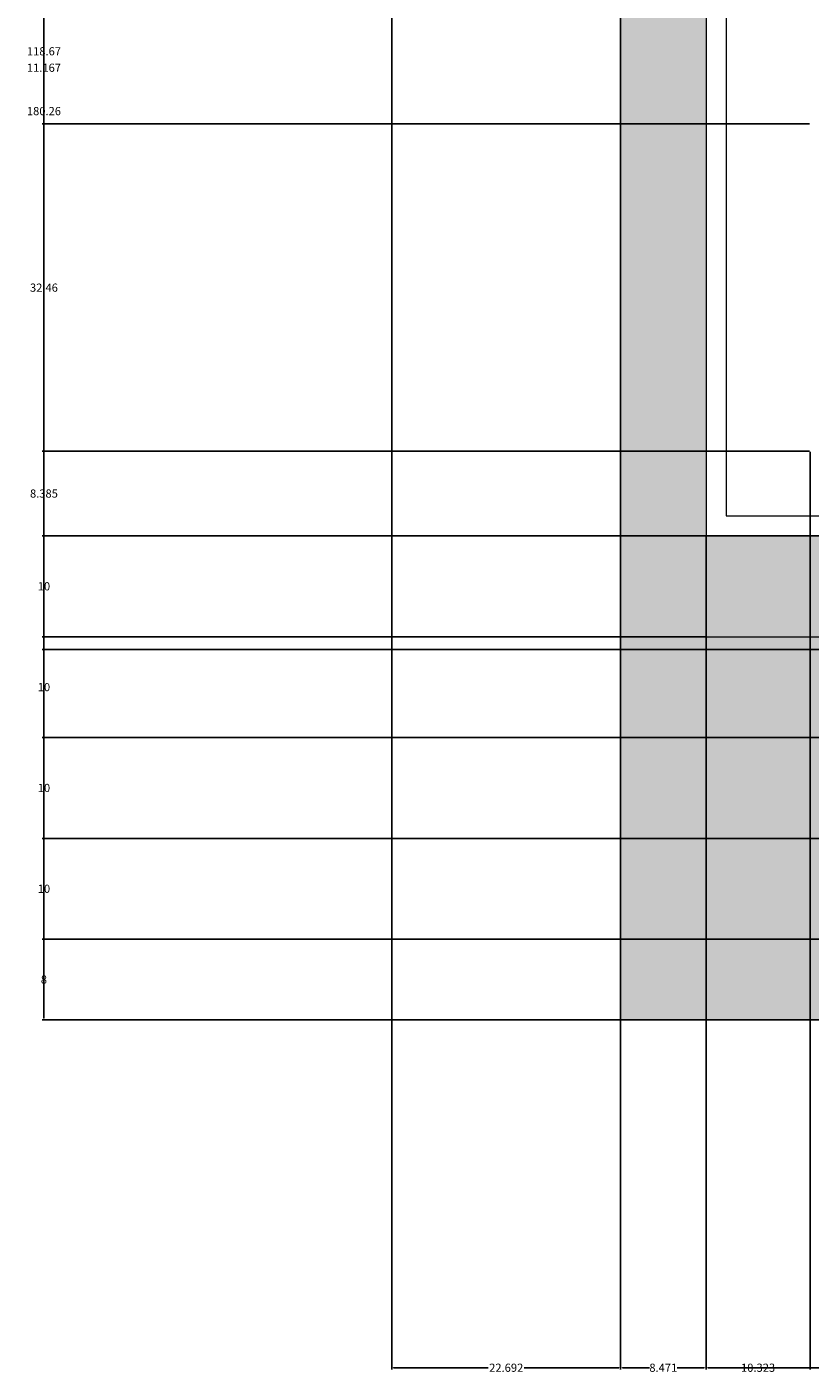
# Model space of a CAD drawing. Units: inches. Extents: x 36 to 594, y 79 to 831.
# Tile 1 of 30: x 36 to 114, y 79 to 213. Entities that reach past the tile are written whole.
import ezdxf

# ---------------------------------------------------------------- set-up
doc = ezdxf.new("R2010")
doc.units = ezdxf.units.IN
doc.header["$MEASUREMENT"] = 0
for name, color, linetype, lineweight in [('A-ANNO-DIMS', 2, 'Continuous', 18), ('A-DOOR', 3, 'Continuous', 18), ('A-ELEV', 7, 'Continuous', 25), ('A-ELEV-PATT', 8, 'Continuous', 13)]:
    doc.layers.add(name, color=color, linetype=linetype, lineweight=lineweight)
doc.styles.get("Standard").update_dxf_attribs({"font": 'arial.ttf'})
doc.dimstyles.get("Standard").update_dxf_attribs({"dimtxt": 0.8125, "dimasz": 0.18, "dimexe": 0.18, "dimexo": 0.0625, "dimgap": 0.09, "dimtad": 0, "dimtih": 1, "dimtoh": 1, "dimdec": 4, "dimzin": 0, "dimdsep": 46, "dimlunit": 4, "dimtxsty": 'Standard', "dimcen": 0.09, "dimadec": 0, "dimazin": 0, "dimtfac": 1, "dimtdec": 4, "dimtofl": 0, "dimtmove": 0, "dimatfit": 3, "dimfxl": 1, "dimtolj": 1, "dimtzin": 0, "dimarcsym": 0})

# ---------------------------------------------------------------- blocks, each defined once
blk = doc.blocks.new('*D7')
at = {"layer": 'A-ANNO-DIMS', "color": 0, "lineweight": -2, "transparency": 16777216}
for p, q in [((94.87, 114.15), (94.87, 79.53)), ((103.34, 114.15), (103.34, 79.53)), ((95.05, 79.71), (97.72, 79.71)), ((103.16, 79.71), (100.48, 79.71))]:
    blk.add_line(p, q, dxfattribs=at)
at = {"layer": 'A-ANNO-DIMS', "color": 0, "transparency": 16777216}
for points in [[(95.05, 79.74), (95.05, 79.68), (94.87, 79.71)], [(103.16, 79.74), (103.16, 79.68), (103.34, 79.71)]]:
    blk.add_solid(points, dxfattribs=at)
at = {"layer": 'Defpoints', "color": 0, "transparency": 16777216}
for p in [(94.87, 114.21), (103.34, 114.21), (103.34, 79.71)]:
    blk.add_point(p, dxfattribs=at)
at = {"layer": 'A-ANNO-DIMS', "color": 0, "transparency": 16777216, "insert": (99.1, 79.71), "char_height": 0.812, "attachment_point": 5}
blk.add_mtext('\\A1;8.471', dxfattribs=at)
blk = doc.blocks.new('*D8')
at = {"layer": 'A-ANNO-DIMS', "color": 0, "lineweight": -2, "transparency": 16777216}
for p, q in [((103.34, 114.15), (103.34, 79.53)), ((217.03, 114.15), (217.03, 79.53)), ((103.52, 79.71), (158.76, 79.71)), ((216.85, 79.71), (161.6, 79.71))]:
    blk.add_line(p, q, dxfattribs=at)
at = {"layer": 'A-ANNO-DIMS', "color": 0, "transparency": 16777216}
for points in [[(103.52, 79.74), (103.52, 79.68), (103.34, 79.71)], [(216.85, 79.74), (216.85, 79.68), (217.03, 79.71)]]:
    blk.add_solid(points, dxfattribs=at)
at = {"layer": 'Defpoints', "color": 0, "transparency": 16777216}
for p in [(103.34, 114.21), (217.03, 114.21), (217.03, 79.71)]:
    blk.add_point(p, dxfattribs=at)
at = {"layer": 'A-ANNO-DIMS', "color": 0, "transparency": 16777216, "insert": (160.18, 79.71), "char_height": 0.812, "attachment_point": 5}
blk.add_mtext('\\A1;113.7', dxfattribs=at)
blk = doc.blocks.new('*D28')
at = {"layer": 'A-ANNO-DIMS', "color": 0, "lineweight": -2, "transparency": 16777216}
for p, q in [((269.3, 796.05), (37.49, 796.05)), ((37.67, 795.87), (37.67, 455.63)), ((37.67, 114.39), (37.67, 454.62)), ((94.8, 114.21), (37.49, 114.21))]:
    blk.add_line(p, q, dxfattribs=at)
at = {"layer": 'A-ANNO-DIMS', "color": 0, "transparency": 16777216}
for points in [[(37.64, 795.87), (37.7, 795.87), (37.67, 796.05)], [(37.64, 114.39), (37.7, 114.39), (37.67, 114.21)]]:
    blk.add_solid(points, dxfattribs=at)
at = {"layer": 'Defpoints', "color": 0, "transparency": 16777216}
for p in [(37.67, 796.05), (269.36, 796.05), (94.87, 114.21)]:
    blk.add_point(p, dxfattribs=at)
at = {"layer": 'A-ANNO-DIMS', "color": 0, "transparency": 16777216, "insert": (37.67, 455.13), "char_height": 0.812, "attachment_point": 5}
blk.add_mtext('\\A1;681.8', dxfattribs=at)
blk = doc.blocks.new('*D42')
at = {"layer": 'A-ANNO-DIMS', "color": 0, "lineweight": -2, "transparency": 16777216}
for p, q in [((72.11, 294.48), (37.49, 294.48)), ((37.67, 294.3), (37.67, 204.85)), ((37.67, 114.39), (37.67, 203.84)), ((94.8, 114.21), (37.49, 114.21))]:
    blk.add_line(p, q, dxfattribs=at)
at = {"layer": 'A-ANNO-DIMS', "color": 0, "transparency": 16777216}
for points in [[(37.64, 294.3), (37.7, 294.3), (37.67, 294.48)], [(37.64, 114.39), (37.7, 114.39), (37.67, 114.21)]]:
    blk.add_solid(points, dxfattribs=at)
at = {"layer": 'Defpoints', "color": 0, "transparency": 16777216}
for p in [(37.67, 294.48), (72.17, 294.48), (94.87, 114.21)]:
    blk.add_point(p, dxfattribs=at)
at = {"layer": 'A-ANNO-DIMS', "color": 0, "transparency": 16777216, "insert": (37.67, 204.34), "char_height": 0.812, "attachment_point": 5}
blk.add_mtext('\\A1;180.26', dxfattribs=at)
blk = doc.blocks.new('*D53')
at = {"layer": 'A-ANNO-DIMS', "color": 0, "lineweight": -2, "transparency": 16777216}
for p, q in [((72.17, 294.41), (72.17, 79.53)), ((94.87, 294.41), (94.87, 79.53)), ((72.35, 79.71), (81.74, 79.71)), ((94.69, 79.71), (85.3, 79.71))]:
    blk.add_line(p, q, dxfattribs=at)
at = {"layer": 'A-ANNO-DIMS', "color": 0, "transparency": 16777216}
for points in [[(72.35, 79.74), (72.35, 79.68), (72.17, 79.71)], [(94.69, 79.74), (94.69, 79.68), (94.87, 79.71)]]:
    blk.add_solid(points, dxfattribs=at)
at = {"layer": 'Defpoints', "color": 0, "transparency": 16777216}
for p in [(72.17, 294.48), (94.87, 294.48), (94.87, 79.71)]:
    blk.add_point(p, dxfattribs=at)
at = {"layer": 'A-ANNO-DIMS', "color": 0, "transparency": 16777216, "insert": (83.52, 79.71), "char_height": 0.812, "attachment_point": 5}
blk.add_mtext('\\A1;22.692', dxfattribs=at)
blk = doc.blocks.new('*D54')
at = {"layer": 'A-ANNO-DIMS', "color": 0, "lineweight": -2, "transparency": 16777216}
for p, q in [((103.27, 122.21), (37.49, 122.21)), ((37.67, 122.03), (37.67, 118.72)), ((37.67, 114.39), (37.67, 117.71)), ((103.27, 114.21), (37.49, 114.21))]:
    blk.add_line(p, q, dxfattribs=at)
at = {"layer": 'A-ANNO-DIMS', "color": 0, "transparency": 16777216}
for points in [[(37.64, 122.03), (37.7, 122.03), (37.67, 122.21)], [(37.64, 114.39), (37.7, 114.39), (37.67, 114.21)]]:
    blk.add_solid(points, dxfattribs=at)
at = {"layer": 'Defpoints', "color": 0, "transparency": 16777216}
for p in [(37.67, 122.21), (103.34, 122.21), (103.34, 114.21)]:
    blk.add_point(p, dxfattribs=at)
at = {"layer": 'A-ANNO-DIMS', "color": 0, "transparency": 16777216, "insert": (37.67, 118.21), "char_height": 0.812, "attachment_point": 5}
blk.add_mtext('\\A1;8', dxfattribs=at)
blk = doc.blocks.new('*D55')
at = {"layer": 'A-ANNO-DIMS', "color": 0, "lineweight": -2, "transparency": 16777216}
for p, q in [((103.27, 132.21), (37.49, 132.21)), ((37.67, 132.03), (37.67, 127.72)), ((37.67, 122.39), (37.67, 126.71)), ((103.27, 122.21), (37.49, 122.21))]:
    blk.add_line(p, q, dxfattribs=at)
at = {"layer": 'A-ANNO-DIMS', "color": 0, "transparency": 16777216}
for points in [[(37.64, 132.03), (37.7, 132.03), (37.67, 132.21)], [(37.64, 122.39), (37.7, 122.39), (37.67, 122.21)]]:
    blk.add_solid(points, dxfattribs=at)
at = {"layer": 'Defpoints', "color": 0, "transparency": 16777216}
for p in [(37.67, 132.21), (103.34, 132.21), (103.34, 122.21)]:
    blk.add_point(p, dxfattribs=at)
at = {"layer": 'A-ANNO-DIMS', "color": 0, "transparency": 16777216, "insert": (37.67, 127.21), "char_height": 0.812, "attachment_point": 5}
blk.add_mtext('\\A1;10', dxfattribs=at)
blk = doc.blocks.new('*D56')
at = {"layer": 'A-ANNO-DIMS', "color": 0, "lineweight": -2, "transparency": 16777216}
for p, q in [((103.27, 142.21), (37.49, 142.21)), ((37.67, 142.03), (37.67, 137.72)), ((37.67, 132.39), (37.67, 136.71)), ((103.27, 132.21), (37.49, 132.21))]:
    blk.add_line(p, q, dxfattribs=at)
at = {"layer": 'A-ANNO-DIMS', "color": 0, "transparency": 16777216}
for points in [[(37.64, 142.03), (37.7, 142.03), (37.67, 142.21)], [(37.64, 132.39), (37.7, 132.39), (37.67, 132.21)]]:
    blk.add_solid(points, dxfattribs=at)
at = {"layer": 'Defpoints', "color": 0, "transparency": 16777216}
for p in [(37.67, 142.21), (103.34, 142.21), (103.34, 132.21)]:
    blk.add_point(p, dxfattribs=at)
at = {"layer": 'A-ANNO-DIMS', "color": 0, "transparency": 16777216, "insert": (37.67, 137.21), "char_height": 0.812, "attachment_point": 5}
blk.add_mtext('\\A1;10', dxfattribs=at)
blk = doc.blocks.new('*D57')
at = {"layer": 'A-ANNO-DIMS', "color": 0, "lineweight": -2, "transparency": 16777216}
for p, q in [((103.27, 152.21), (37.49, 152.21)), ((37.67, 152.03), (37.67, 147.72)), ((37.67, 142.39), (37.67, 146.71)), ((103.27, 142.21), (37.49, 142.21))]:
    blk.add_line(p, q, dxfattribs=at)
at = {"layer": 'A-ANNO-DIMS', "color": 0, "transparency": 16777216}
for points in [[(37.64, 152.03), (37.7, 152.03), (37.67, 152.21)], [(37.64, 142.39), (37.7, 142.39), (37.67, 142.21)]]:
    blk.add_solid(points, dxfattribs=at)
at = {"layer": 'Defpoints', "color": 0, "transparency": 16777216}
for p in [(37.67, 152.21), (103.34, 152.21), (103.34, 142.21)]:
    blk.add_point(p, dxfattribs=at)
at = {"layer": 'A-ANNO-DIMS', "color": 0, "transparency": 16777216, "insert": (37.67, 147.21), "char_height": 0.812, "attachment_point": 5}
blk.add_mtext('\\A1;10', dxfattribs=at)
blk = doc.blocks.new('*D58')
at = {"layer": 'A-ANNO-DIMS', "color": 0, "lineweight": -2, "transparency": 16777216}
for p, q in [((103.27, 162.21), (37.49, 162.21)), ((37.67, 162.03), (37.67, 157.72)), ((37.67, 152.39), (37.67, 156.71)), ((103.27, 152.21), (37.49, 152.21))]:
    blk.add_line(p, q, dxfattribs=at)
at = {"layer": 'A-ANNO-DIMS', "color": 0, "transparency": 16777216}
for points in [[(37.64, 162.03), (37.7, 162.03), (37.67, 162.21)], [(37.64, 152.39), (37.7, 152.39), (37.67, 152.21)]]:
    blk.add_solid(points, dxfattribs=at)
at = {"layer": 'Defpoints', "color": 0, "transparency": 16777216}
for p in [(37.67, 162.21), (103.34, 162.21), (103.34, 152.21)]:
    blk.add_point(p, dxfattribs=at)
at = {"layer": 'A-ANNO-DIMS', "color": 0, "transparency": 16777216, "insert": (37.67, 157.21), "char_height": 0.812, "attachment_point": 5}
blk.add_mtext('\\A1;10', dxfattribs=at)
blk = doc.blocks.new('*D62')
at = {"layer": 'A-ANNO-DIMS', "color": 0, "lineweight": -2, "transparency": 16777216}
for p, q in [((113.66, 170.54), (113.66, 79.53)), ((103.34, 162.15), (103.34, 79.53)), ((103.52, 79.71), (106.76, 79.71)), ((113.48, 79.71), (110.24, 79.71))]:
    blk.add_line(p, q, dxfattribs=at)
at = {"layer": 'A-ANNO-DIMS', "color": 0, "transparency": 16777216}
for points in [[(103.52, 79.74), (103.52, 79.68), (103.34, 79.71)], [(113.48, 79.74), (113.48, 79.68), (113.66, 79.71)]]:
    blk.add_solid(points, dxfattribs=at)
at = {"layer": 'Defpoints', "color": 0, "transparency": 16777216}
for p in [(113.66, 170.6), (103.34, 162.21), (113.66, 79.71)]:
    blk.add_point(p, dxfattribs=at)
at = {"layer": 'A-ANNO-DIMS', "color": 0, "transparency": 16777216, "insert": (108.5, 79.71), "char_height": 0.812, "attachment_point": 5}
blk.add_mtext('\\A1;10.323', dxfattribs=at)
blk = doc.blocks.new('*D63')
at = {"layer": 'A-ANNO-DIMS', "color": 0, "lineweight": -2, "transparency": 16777216}
for p, q in [((113.66, 170.54), (113.66, 79.53)), ((148.04, 170.54), (148.04, 79.53)), ((113.84, 79.71), (129.39, 79.71)), ((147.86, 79.71), (132.31, 79.71))]:
    blk.add_line(p, q, dxfattribs=at)
at = {"layer": 'A-ANNO-DIMS', "color": 0, "transparency": 16777216}
for points in [[(113.84, 79.74), (113.84, 79.68), (113.66, 79.71)], [(147.86, 79.74), (147.86, 79.68), (148.04, 79.71)]]:
    blk.add_solid(points, dxfattribs=at)
at = {"layer": 'Defpoints', "color": 0, "transparency": 16777216}
for p in [(113.66, 170.6), (148.04, 170.6), (148.04, 79.71)]:
    blk.add_point(p, dxfattribs=at)
at = {"layer": 'A-ANNO-DIMS', "color": 0, "transparency": 16777216, "insert": (130.85, 79.71), "char_height": 0.812, "attachment_point": 5}
blk.add_mtext('\\A1;34.38', dxfattribs=at)
blk = doc.blocks.new('*D68')
at = {"layer": 'A-ANNO-DIMS', "color": 0, "lineweight": -2, "transparency": 16777216}
for p, q in [((113.6, 170.6), (37.49, 170.6)), ((37.67, 170.42), (37.67, 166.91)), ((37.67, 162.39), (37.67, 165.9)), ((103.27, 162.21), (37.49, 162.21))]:
    blk.add_line(p, q, dxfattribs=at)
at = {"layer": 'A-ANNO-DIMS', "color": 0, "transparency": 16777216}
for points in [[(37.64, 170.42), (37.7, 170.42), (37.67, 170.6)], [(37.64, 162.39), (37.7, 162.39), (37.67, 162.21)]]:
    blk.add_solid(points, dxfattribs=at)
at = {"layer": 'Defpoints', "color": 0, "transparency": 16777216}
for p in [(37.67, 170.6), (113.66, 170.6), (103.34, 162.21)]:
    blk.add_point(p, dxfattribs=at)
at = {"layer": 'A-ANNO-DIMS', "color": 0, "transparency": 16777216, "insert": (37.67, 166.41), "char_height": 0.812, "attachment_point": 5}
blk.add_mtext('\\A1;8.385', dxfattribs=at)
blk = doc.blocks.new('*D69')
at = {"layer": 'A-ANNO-DIMS', "color": 0, "lineweight": -2, "transparency": 16777216}
for p, q in [((113.6, 203.06), (37.49, 203.06)), ((37.67, 202.88), (37.67, 187.33)), ((37.67, 170.78), (37.67, 186.32)), ((113.6, 170.6), (37.49, 170.6))]:
    blk.add_line(p, q, dxfattribs=at)
at = {"layer": 'A-ANNO-DIMS', "color": 0, "transparency": 16777216}
for points in [[(37.64, 202.88), (37.7, 202.88), (37.67, 203.06)], [(37.64, 170.78), (37.7, 170.78), (37.67, 170.6)]]:
    blk.add_solid(points, dxfattribs=at)
at = {"layer": 'Defpoints', "color": 0, "transparency": 16777216}
for p in [(37.67, 203.06), (113.66, 203.06), (113.66, 170.6)]:
    blk.add_point(p, dxfattribs=at)
at = {"layer": 'A-ANNO-DIMS', "color": 0, "transparency": 16777216, "insert": (37.67, 186.83), "char_height": 0.812, "attachment_point": 5}
blk.add_mtext('\\A1;32.46', dxfattribs=at)
blk = doc.blocks.new('*D70')
at = {"layer": 'A-ANNO-DIMS', "color": 0, "lineweight": -2, "transparency": 16777216}
for p, q in [((113.6, 214.22), (37.49, 214.22)), ((37.67, 214.04), (37.67, 209.15)), ((37.67, 203.24), (37.67, 208.14)), ((113.6, 203.06), (37.49, 203.06))]:
    blk.add_line(p, q, dxfattribs=at)
at = {"layer": 'A-ANNO-DIMS', "color": 0, "transparency": 16777216}
for points in [[(37.64, 214.04), (37.7, 214.04), (37.67, 214.22)], [(37.64, 203.24), (37.7, 203.24), (37.67, 203.06)]]:
    blk.add_solid(points, dxfattribs=at)
at = {"layer": 'Defpoints', "color": 0, "transparency": 16777216}
for p in [(37.67, 214.22), (113.66, 214.22), (113.66, 203.06)]:
    blk.add_point(p, dxfattribs=at)
at = {"layer": 'A-ANNO-DIMS', "color": 0, "transparency": 16777216, "insert": (37.67, 208.64), "char_height": 0.812, "attachment_point": 5}
blk.add_mtext('\\A1;11.167', dxfattribs=at)
blk = doc.blocks.new('*D90')
at = {"layer": 'A-ANNO-DIMS', "color": 0, "lineweight": -2, "transparency": 16777216}
for p, q in [((255.97, 269.61), (37.49, 269.61)), ((37.67, 269.43), (37.67, 210.78)), ((37.67, 151.11), (37.67, 209.77)), ((253.97, 150.93), (37.49, 150.93))]:
    blk.add_line(p, q, dxfattribs=at)
at = {"layer": 'A-ANNO-DIMS', "color": 0, "transparency": 16777216}
for points in [[(37.64, 269.43), (37.7, 269.43), (37.67, 269.61)], [(37.64, 151.11), (37.7, 151.11), (37.67, 150.93)]]:
    blk.add_solid(points, dxfattribs=at)
at = {"layer": 'Defpoints', "color": 0, "transparency": 16777216}
for p in [(37.67, 269.61), (256.03, 269.61), (254.03, 150.93)]:
    blk.add_point(p, dxfattribs=at)
at = {"layer": 'A-ANNO-DIMS', "color": 0, "transparency": 16777216, "insert": (37.67, 210.27), "char_height": 0.812, "attachment_point": 5}
blk.add_mtext('\\A1;118.67', dxfattribs=at)

msp = doc.modelspace()

# ---------------------------------------------------------------- hatches: boundary and pattern name
at = {"layer": 'A-ELEV-PATT'}
h = msp.add_hatch(color=256, dxfattribs=at)
h.dxf.hatch_style = 1
h.paths.add_polyline_path([(398.0873, 796.0465), (269.3592, 796.0465), (269.3592, 770.1455), (397.8159, 770.1455)])
h.paths.add_polyline_path([(397.7518, 764.0341), (269.3592, 764.0341), (269.3592, 630.0394), (341.8367, 630.0394), (341.8367, 720.595), (335.0881, 728.3699), (329.982, 735.3373), (345.3661, 727.7743), (397.1052, 702.3389)])
h.paths.add_polyline_path([(341.8367, 594.2124), (201.4189, 594.2124), (201.4189, 475.4136), (232.8216, 475.4136), (232.8216, 524.6037), (341.8367, 524.6037)])
h.paths.add_polyline_path([(177.525, 594.2124), (118.7598, 594.2124), (118.7598, 450.2124), (177.525, 450.2124)])
h.paths.add_polyline_path([(424.4958, 594.2124), (365.7306, 594.2124), (365.7306, 450.2124), (424.4958, 450.2124)])
h.paths.add_polyline_path([(241.3553, 404.2737), (355.8569, 404.2737), (355.8569, 355.0836), (424.5492, 355.0836), (424.5492, 425.7333), (118.7598, 426.2844), (118.7598, 355.0836), (241.3553, 355.0836)])
h.paths.add_polyline_path([(448.3898, 306.2124), (217.0273, 306.2124), (217.0273, 142.2124), (254.0293, 142.2124), (254.0293, 150.9347), (254.0293, 286.1802), (401.5491, 286.1802), (401.5491, 150.9347), (401.5491, 142.2124), (448.3898, 142.2124)])
h.paths.add_polyline_path([(448.3898, 142.2124), (401.5491, 142.2124), (217.0273, 142.2124), (217.0273, 114.2124), (448.3898, 114.2124)])
h.paths.add_polyline_path([(217.0273, 306.2124), (174.7353, 306.2124), (94.8658, 306.2124), (94.8658, 162.2124), (103.3368, 162.2124), (103.3368, 264.6224), (103.3368, 286.1802), (217.0273, 286.1802)])
h = msp.add_hatch(color=256, dxfattribs=at)
h.dxf.hatch_style = 1
h.set_gradient(color1=(192, 192, 192), color2=(0, 0, 0))
h.paths.add_polyline_path([(243.19, 469.3251), (222.9132, 469.3251), (222.9132, 454.5571), (243.1634, 454.5571)])
h.paths.add_polyline_path([(264.4667, 469.2868), (244.1899, 469.2868), (244.1899, 454.5188), (264.4401, 454.5188)])
h.paths.add_polyline_path([(285.7435, 469.2484), (265.4667, 469.2484), (265.4667, 454.4804), (285.7168, 454.4804)])
h.paths.add_polyline_path([(307.0202, 469.2101), (286.7434, 469.2101), (286.7434, 454.4421), (306.9936, 454.4421)])
h.paths.add_polyline_path([(328.2969, 469.1717), (308.0201, 469.1717), (308.0201, 454.4037), (328.2703, 454.4037)])
h.paths.add_polyline_path([(341.8367, 469.1334), (329.2969, 469.1334), (329.2969, 454.3654), (341.8367, 454.3654)])
h.paths.add_polyline_path([(221.9133, 469.3635), (201.6365, 469.3635), (201.6365, 454.5955), (221.8866, 454.5955)])
h.paths.add_polyline_path([(145.3401, 349.1868), (125.0633, 349.1868), (125.0633, 334.4189), (145.3134, 334.4189)])
h.paths.add_polyline_path([(166.6168, 349.1485), (146.34, 349.1485), (146.34, 334.3805), (166.5902, 334.3805)])
h.paths.add_polyline_path([(187.8935, 349.1101), (167.6167, 349.1101), (167.6167, 334.3422), (187.8669, 334.3422)])
h.paths.add_polyline_path([(209.1703, 349.0718), (188.8935, 349.0718), (188.8935, 334.3038), (209.1436, 334.3038)])
h.paths.add_polyline_path([(230.447, 349.0335), (210.1702, 349.0335), (210.1702, 334.2655), (230.4204, 334.2655)])
h.paths.add_polyline_path([(251.7237, 348.9951), (231.4469, 348.9951), (231.4469, 334.2271), (251.6971, 334.2271)])
h.paths.add_polyline_path([(273.0005, 348.9568), (252.7236, 348.9568), (252.7236, 334.1888), (272.9738, 334.1888)])
h.paths.add_polyline_path([(294.2772, 348.9184), (274.0004, 348.9184), (274.0004, 334.1504), (294.2506, 334.1504)])
h.paths.add_polyline_path([(315.5539, 348.8801), (295.2771, 348.8801), (295.2771, 334.1121), (315.5273, 334.1121)])
h.paths.add_polyline_path([(336.8306, 348.8417), (316.5538, 348.8417), (316.5538, 334.0737), (336.804, 334.0737)])
h.paths.add_polyline_path([(358.1074, 348.8034), (337.8306, 348.8034), (337.8306, 334.0354), (358.0808, 334.0354)])
h.paths.add_polyline_path([(379.3841, 348.765), (359.1073, 348.765), (359.1073, 333.997), (379.3575, 333.997)])
h.paths.add_polyline_path([(400.6608, 348.7267), (380.384, 348.7267), (380.384, 333.9587), (400.6342, 333.9587)])
h.paths.add_polyline_path([(421.9376, 348.6883), (401.6608, 348.6883), (401.6608, 333.9204), (421.911, 333.9204)])
h.paths.add_polyline_path([(103.3368, 162.2124), (94.8658, 162.2124), (94.8658, 150.2124), (94.8658, 114.2124), (103.3368, 114.2124)])
h.paths.add_polyline_path([(217.0273, 132.2124), (103.3368, 132.2124), (103.3368, 122.2124), (217.0273, 122.2124)])
h.paths.add_polyline_path([(217.0273, 122.2124), (103.3368, 122.2124), (103.3368, 114.2124), (217.0273, 114.2124)])
h.paths.add_polyline_path([(217.0273, 142.2124), (174.7353, 142.2124), (103.3368, 142.2124), (103.3368, 132.2124), (217.0273, 132.2124)])
h.paths.add_polyline_path([(217.0273, 152.2124), (103.3368, 152.2124), (103.3368, 142.2124), (174.7353, 142.2124), (217.0273, 142.2124)])
h.paths.add_polyline_path([(217.0273, 162.2124), (103.3368, 162.2124), (103.3368, 152.2124), (217.0273, 152.2124)])

# ---------------------------------------------------------------- linework, layer by layer
at = {"layer": 'A-DOOR'}
msp.add_line((103.3368, 152.2124), (217.0273, 152.2124), dxfattribs=at)
for points in [[(103.3368, 162.2124), (156.4069, 162.2124), (156.4069, 264.6224), (103.3368, 264.6224)], [(105.3368, 164.2124), (154.4069, 164.2124), (154.4069, 262.6224), (105.3368, 262.6224)]]:
    msp.add_lwpolyline(points, close=True, dxfattribs=at)
at = {"layer": 'A-ELEV'}
for p, q in [((94.8658, 162.2124), (94.8658, 306.2124)), ((94.8658, 150.2124), (94.8658, 162.2124)), ((94.8658, 162.2124), (217.0273, 162.2124)), ((103.3368, 162.2124), (103.3368, 114.2124)), ((94.8658, 114.2124), (94.8658, 150.2124)), ((103.3368, 142.2124), (174.7353, 142.2124)), ((103.3368, 132.2124), (217.0273, 132.2124)), ((103.3368, 122.2124), (217.0273, 122.2124)), ((84.3711, 114.2124), (558.1689, 114.2124))]:
    msp.add_line(p, q, dxfattribs=at)

# ---------------------------------------------------------------- dimensions: what is measured, and where the dimension line sits
at = {"layer": 'A-ANNO-DIMS'}
for base, p1, p2, override, picture, middle in [((37.6733, 796.0465), (94.8658, 114.2124), (269.3592, 796.0465), {"dimdec": 1, "dimlfac": 1, "dimrnd": 0, "dimzin": 0, "dimdsep": 46, "dimlunit": 2}, '*D28', (37.6733, 455.1294)), ((37.6733, 294.4759), (94.8658, 114.2124), (72.1733, 294.4759), {"dimdec": 2, "dimlfac": 1, "dimrnd": 0, "dimzin": 0, "dimdsep": 46, "dimlunit": 2}, '*D42', (37.6733, 204.3442)), ((37.6733, 269.6084), (254.0293, 150.9347), (256.0293, 269.6084), {"dimdec": 2, "dimlfac": 1, "dimrnd": 0, "dimzin": 0, "dimdsep": 46, "dimlunit": 2}, '*D90', (37.6733, 210.2716)), ((37.6733, 214.2237), (113.6593, 203.057), (113.6593, 214.2237), {"dimdec": 3, "dimlfac": 1, "dimrnd": 0, "dimzin": 0, "dimdsep": 46, "dimlunit": 2}, '*D70', (37.6733, 208.6404)), ((37.6733, 203.057), (113.6593, 170.5978), (113.6593, 203.057), {"dimdec": 2, "dimlfac": 1, "dimrnd": 0, "dimzin": 0, "dimdsep": 46, "dimlunit": 2}, '*D69', (37.6733, 186.8274)), ((37.6733, 170.5978), (103.3368, 162.2124), (113.6593, 170.5978), {"dimdec": 3, "dimlfac": 1, "dimrnd": 0, "dimzin": 0, "dimdsep": 46, "dimlunit": 2}, '*D68', (37.6733, 166.4051)), ((37.6733, 162.2124), (103.3368, 152.2124), (103.3368, 162.2124), {"dimdec": 0, "dimlfac": 1, "dimrnd": 0, "dimzin": 0, "dimdsep": 46, "dimlunit": 2}, '*D58', (37.6733, 157.2124)), ((37.6733, 152.2124), (103.3368, 142.2124), (103.3368, 152.2124), {"dimdec": 0, "dimlfac": 1, "dimrnd": 0, "dimzin": 0, "dimdsep": 46, "dimlunit": 2}, '*D57', (37.6733, 147.2124)), ((37.6733, 142.2124), (103.3368, 132.2124), (103.3368, 142.2124), {"dimdec": 0, "dimlfac": 1, "dimrnd": 0, "dimzin": 0, "dimdsep": 46, "dimlunit": 2}, '*D56', (37.6733, 137.2124)), ((37.6733, 132.2124), (103.3368, 122.2124), (103.3368, 132.2124), {"dimdec": 0, "dimlfac": 1, "dimrnd": 0, "dimzin": 0, "dimdsep": 46, "dimlunit": 2}, '*D55', (37.6733, 127.2124)), ((37.6733, 122.2124), (103.3368, 114.2124), (103.3368, 122.2124), {"dimdec": 0, "dimlfac": 1, "dimrnd": 0, "dimzin": 0, "dimdsep": 46, "dimlunit": 2}, '*D54', (37.6733, 118.2124))]:
    dim = msp.add_linear_dim(base=base, p1=p1, p2=p2, angle=90, dimstyle='Standard', override=override, dxfattribs=at)
    dim.commit()
    dim.dimension.update_dxf_attribs({"geometry": picture, "text_midpoint": middle})
for base, p1, p2, override, picture, middle in [((94.86583, 79.71236), (72.17334, 294.47595), (94.86583, 294.47595), {"dimdec": 3, "dimlfac": 1, "dimrnd": 0, "dimzin": 0, "dimdsep": 46, "dimlunit": 2}, '*D53', (83.51959, 79.71236)), ((113.65927, 79.71236), (103.33676, 162.21236), (113.65927, 170.5978), {"dimdec": 3, "dimlfac": 1, "dimrnd": 0, "dimzin": 0, "dimdsep": 46, "dimlunit": 2}, '*D62', (108.49802, 79.71236)), ((148.0383, 79.7124), (113.6593, 170.5978), (148.0383, 170.5978), {"dimdec": 2, "dimlfac": 1, "dimrnd": 0, "dimzin": 0, "dimdsep": 46, "dimlunit": 2}, '*D63', (130.8488, 79.7124)), ((103.3368, 79.7124), (94.8658, 114.2124), (103.3368, 114.2124), {"dimdec": 3, "dimlfac": 1, "dimrnd": 0, "dimzin": 0, "dimdsep": 46, "dimlunit": 2}, '*D7', (99.1013, 79.7124)), ((217.0273, 79.7124), (103.3368, 114.2124), (217.0273, 114.2124), {"dimdec": 1, "dimlfac": 1, "dimrnd": 0, "dimzin": 0, "dimdsep": 46, "dimlunit": 2}, '*D8', (160.182, 79.7124))]:
    dim = msp.add_linear_dim(base=base, p1=p1, p2=p2, dimstyle='Standard', override=override, dxfattribs=at)
    dim.commit()
    dim.dimension.update_dxf_attribs({"geometry": picture, "text_midpoint": middle})

doc.saveas('drawing.dxf')
